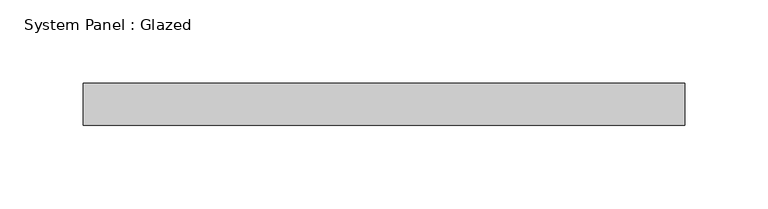
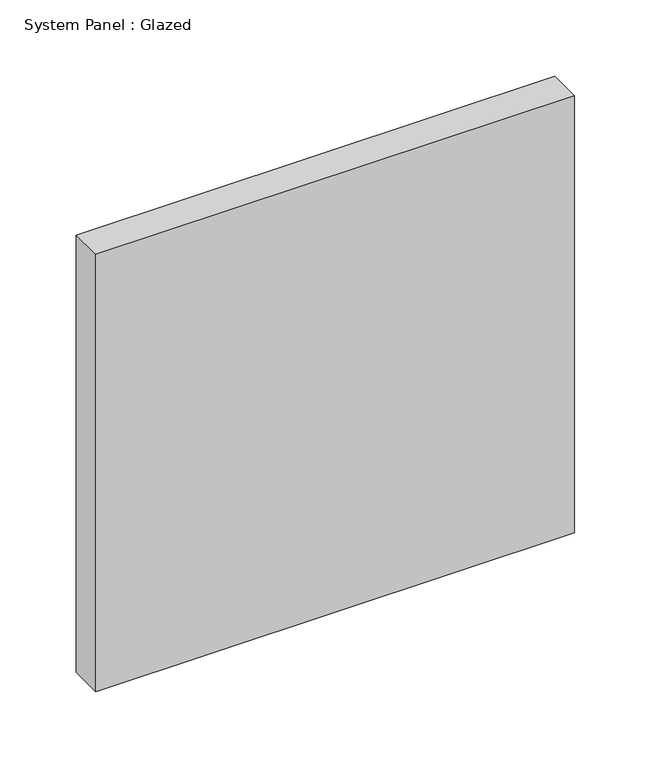
"""IFC4 building model written with IfcOpenShell, lengths in millimetres: plate geometry, System Panel : Glazed."""

from ifc_helpers import new_model, si_unit, origin, origin_with_axes, place, context, project, spatial, polyline, outline, extrude, source, transform, mapped, element, save


def system_panel_glazed_6a2c27ee(model_context):
    return source(origin(), model_context, "Body", "SweptSolid", [
        extrude(outline(polyline([(180.975, 19.05), (-180.975, 19.05), (-180.975, 44.45), (180.975, 44.45), (180.975, 19.05)])), origin_with_axes(), (0.0, 0.0, 1.0), 349.25),
    ])


if __name__ == "__main__":
    model = new_model("IFC4")
    model_context = context("Model", 3, world=origin())
    ifc_project = project(units=[si_unit("LENGTHUNIT", "METRE", prefix="MILLI")], contexts=[model_context])
    site = spatial("IfcSite", under=ifc_project)
    building = spatial("IfcBuilding", under=site)
    placement = place(None, origin())
    system_panel_glazed_shape = system_panel_glazed_6a2c27ee(model_context)
    element("IfcPlate", 1, ObjectType="System Panel : Glazed", at=placement, inside=building, context=model_context, shape_type="MappedRepresentation", body=[
        mapped(system_panel_glazed_shape, transform((0.0, 0.0, 0.0), x_axis=(1.0, 0.0, 0.0), y_axis=(0.0, 1.0, 0.0), z_axis=(0.0, 0.0, 1.0))),
    ])
    save(model, "model.ifc")

# Revit data of these elements
# Type "System Panel : Glazed"
#   Construction Type Id = "GSP4R"
#   Analytic Construction = "1/8 in Pilkington single glazing"
#   Visual Light Transmittance = 0.9
#   Solar Heat Gain Coefficient = 0.86
#   Heat Transfer Coefficient (U) = 1.18115 BTU/(h·ft²·°F)
#   Define Thermal Properties by = 1
# Element 1 (IfcPlate, "System Panel : Glazed")
#   Materials on its faces: "Glass"
# Materials
#   "Glass": class "Glass", colour RGB 0 128 192, transparency 0.75, Description = "Soda Lime Glass", Cost = 0
